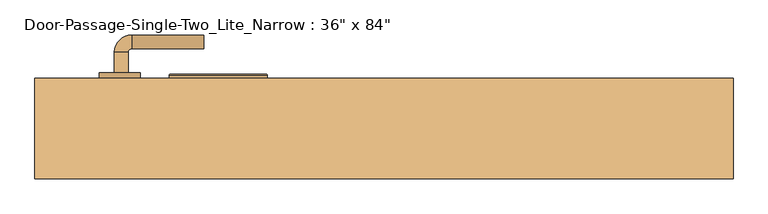
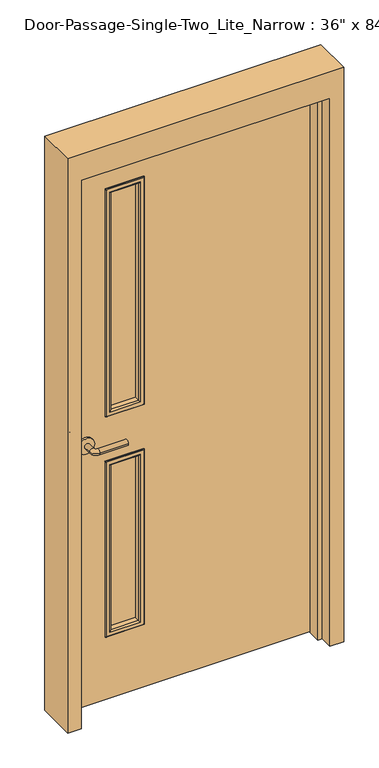
"""IFC4 building model written with IfcOpenShell, lengths in millimetres: door geometry."""

from ifc_helpers import new_model, si_unit, point, frame, frame_2d, origin, place, context, project, spatial, polyline, circle_curve, ellipse_curve, trimmed, segment, composite_curve, outline, extrude, faceted_brep, source, transform, mapped, element, save
from ifc_brep_helpers import plane_surface, cylinder_surface, revolved_surface, advanced_brep


def door_1568ef6f(model_context):
    return source(origin(), model_context, "Body", "SolidModel", [
        advanced_brep(
        [(-392.190625, 4.7, 1016.0), (-372.190625, 4.7, 1016.0), (-372.190625, -25.3, 1016.0), (-392.190625, -25.3, 1016.0), (-367.190625, -30.3, 1016.0), (-367.190625, -50.3, 1016.0), (-262.190625, -50.3, 1016.0), (-262.190625, -30.3, 1016.0)],
        [
            (0, 1, circle_curve(frame((-382.190625, 4.7, 1016.0), z_axis=(0.0, 1.0, 0.0), x_axis=(1.0, 0.0, 0.0)), 10.0)),
            (1, 0, circle_curve(frame((-382.190625, 4.7, 1016.0), z_axis=(0.0, 1.0, 0.0), x_axis=(1.0, 0.0, 0.0)), 10.0)),
            (1, 2),
            (2, 3, circle_curve(frame((-382.190625, -25.3, 1016.0), z_axis=(0.0, 1.0, 0.0), x_axis=(1.0, 0.0, 0.0)), 10.0)),
            (3, 0),
            (3, 2, circle_curve(frame((-382.190625, -25.3, 1016.0), z_axis=(0.0, 1.0, 0.0), x_axis=(1.0, 0.0, 0.0)), 10.0)),
            (4, 5, circle_curve(frame((-367.190625, -40.3, 1016.0), z_axis=(-1.0, 0.0, 0.0), x_axis=(0.0, 1.0, 0.0)), 10.0)),
            (5, 3, circle_curve(frame((-367.190625, -25.3, 1016.0), z_axis=(0.0, 0.0, -1.0), x_axis=(-1.0, 0.0, 0.0)), 25.0)),
            (2, 4, circle_curve(frame((-367.190625, -25.3, 1016.0), z_axis=(0.0, 0.0, 1.0), x_axis=(-1.0, 0.0, 0.0)), 5.0)),
            (5, 4, circle_curve(frame((-367.190625, -40.3, 1016.0), z_axis=(-1.0, 0.0, 0.0), x_axis=(0.0, 1.0, 0.0)), 10.0)),
            (6, 7, circle_curve(frame((-262.190625, -40.3, 1016.0), z_axis=(1.0, 0.0, 0.0), x_axis=(0.0, 1.0, 0.0)), 10.0)),
            (7, 6, circle_curve(frame((-262.190625, -40.3, 1016.0), z_axis=(1.0, 0.0, 0.0), x_axis=(0.0, 1.0, 0.0)), 10.0)),
            (4, 7),
            (6, 5),
        ],
        [
            plane_surface(frame((-382.190625, 4.7, 1016.0), z_axis=(0.0, 1.0, 0.0), x_axis=(0.0, 0.0, 1.0))),
            cylinder_surface(frame((-382.190625, 4.7, 1016.0), z_axis=(0.0, 1.0, 0.0), x_axis=(1.0, 0.0, 0.0)), 10.0),
            revolved_surface(trimmed(ellipse_curve(frame((-382.190625, -25.3, 1016.0), z_axis=(0.0, -1.0, 0.0), x_axis=(1.0, 0.0, 0.0)), 10.0, 10.0), [point((-392.190625, -25.3, 1016.0))], [point((-372.190625, -25.3, 1016.0))], True, "CARTESIAN"), (-367.190625, -25.3, 1016.0), (0.0, 0.0, -1.0)),
            revolved_surface(trimmed(ellipse_curve(frame((-382.190625, -25.3, 1016.0), z_axis=(0.0, -1.0, 0.0), x_axis=(1.0, 0.0, 0.0)), 10.0, 10.0), [point((-372.190625, -25.3, 1016.0))], [point((-392.190625, -25.3, 1016.0))], True, "CARTESIAN"), (-367.190625, -25.3, 1016.0), (0.0, 0.0, -1.0)),
            plane_surface(frame((-262.190625, -40.3, 1016.0), z_axis=(1.0, 0.0, 0.0), x_axis=(0.0, 0.0, 1.0))),
            cylinder_surface(frame((-367.190625, -40.3, 1016.0), z_axis=(-1.0, 0.0, 0.0), x_axis=(0.0, 1.0, 0.0)), 10.0),
        ],
        [
            (0, [[1, 2]]),
            (1, [[3, 4, 5, -2]]),
            (1, [[-5, 6, -3, -1]]),
            (2, [[7, 8, -4, 9]]),
            (3, [[10, -9, -6, -8]]),
            (4, [[11, 12]]),
            (5, [[13, -11, 14, -7]]),
            (5, [[-14, -12, -13, -10]]),
        ],
    ),
        extrude(outline(composite_curve([segment(trimmed(circle_curve(frame_2d((1016.0, -384.690625)), 30.0), [point((1016.0, -414.690625))], [point((1016.0, -354.690625))], False, "CARTESIAN"), True, "CONTINUOUS"), segment(trimmed(circle_curve(frame_2d((1016.0, -384.690625)), 30.0), [point((1016.0, -354.690625))], [point((1016.0, -414.690625))], False, "CARTESIAN"), True, "CONTINUOUS")], self_intersect=False)), frame((0.0, 4.7, 0.0), z_axis=(0.0, 1.0, 0.0), x_axis=(0.0, 0.0, 1.0)), (0.0, 0.0, 1.0), 8.0),
        advanced_brep(
        [(-392.190625, 65.15, 1016.0), (-372.190625, 65.15, 1016.0), (-392.190625, 95.15, 1016.0), (-372.190625, 95.15, 1016.0), (-367.190625, 100.15, 1016.0), (-367.190625, 120.15, 1016.0), (-262.190625, 120.15, 1016.0), (-262.190625, 100.15, 1016.0)],
        [
            (0, 1, circle_curve(frame((-382.190625, 65.15, 1016.0), z_axis=(0.0, -1.0, 0.0), x_axis=(1.0, 0.0, 0.0)), 10.0)),
            (1, 0, circle_curve(frame((-382.190625, 65.15, 1016.0), z_axis=(0.0, -1.0, 0.0), x_axis=(1.0, 0.0, 0.0)), 10.0)),
            (0, 2),
            (2, 3, circle_curve(frame((-382.190625, 95.15, 1016.0), z_axis=(0.0, -1.0, 0.0), x_axis=(1.0, 0.0, 0.0)), 10.0)),
            (3, 1),
            (3, 2, circle_curve(frame((-382.190625, 95.15, 1016.0), z_axis=(0.0, -1.0, 0.0), x_axis=(1.0, 0.0, 0.0)), 10.0)),
            (4, 3, circle_curve(frame((-367.190625, 95.15, 1016.0), z_axis=(0.0, 0.0, 1.0), x_axis=(-1.0, 0.0, 0.0)), 5.0)),
            (2, 5, circle_curve(frame((-367.190625, 95.15, 1016.0), z_axis=(0.0, 0.0, -1.0), x_axis=(-1.0, 0.0, 0.0)), 25.0)),
            (5, 4, circle_curve(frame((-367.190625, 110.15, 1016.0), z_axis=(-1.0, 0.0, 0.0), x_axis=(0.0, -1.0, 0.0)), 10.0)),
            (4, 5, circle_curve(frame((-367.190625, 110.15, 1016.0), z_axis=(-1.0, 0.0, 0.0), x_axis=(0.0, -1.0, 0.0)), 10.0)),
            (6, 7, circle_curve(frame((-262.190625, 110.15, 1016.0), z_axis=(1.0, 0.0, 0.0), x_axis=(0.0, -1.0, 0.0)), 10.0)),
            (7, 6, circle_curve(frame((-262.190625, 110.15, 1016.0), z_axis=(1.0, 0.0, 0.0), x_axis=(0.0, -1.0, 0.0)), 10.0)),
            (5, 6),
            (7, 4),
        ],
        [
            plane_surface(frame((-382.190625, 65.15, 1016.0), z_axis=(0.0, -1.0, 0.0), x_axis=(0.0, 0.0, 1.0))),
            cylinder_surface(frame((-382.190625, 65.15, 1016.0), z_axis=(0.0, -1.0, 0.0), x_axis=(1.0, 0.0, 0.0)), 10.0),
            revolved_surface(trimmed(ellipse_curve(frame((-382.190625, 95.15, 1016.0), z_axis=(0.0, -1.0, 0.0), x_axis=(1.0, 0.0, 0.0)), 10.0, 10.0), [point((-392.190625, 95.15, 1016.0))], [point((-372.190625, 95.15, 1016.0))], True, "CARTESIAN"), (-367.190625, 95.15, 1016.0), (0.0, 0.0, -1.0)),
            revolved_surface(trimmed(ellipse_curve(frame((-382.190625, 95.15, 1016.0), z_axis=(0.0, -1.0, 0.0), x_axis=(1.0, 0.0, 0.0)), 10.0, 10.0), [point((-372.190625, 95.15, 1016.0))], [point((-392.190625, 95.15, 1016.0))], True, "CARTESIAN"), (-367.190625, 95.15, 1016.0), (0.0, 0.0, -1.0)),
            plane_surface(frame((-262.190625, 110.15, 1016.0), z_axis=(1.0, 0.0, 0.0), x_axis=(0.0, 0.0, 1.0))),
            cylinder_surface(frame((-367.190625, 110.15, 1016.0), z_axis=(-1.0, 0.0, 0.0), x_axis=(0.0, -1.0, 0.0)), 10.0),
        ],
        [
            (0, [[1, 2]]),
            (1, [[-1, 3, 4, 5]]),
            (1, [[-2, -5, 6, -3]]),
            (2, [[7, -4, 8, 9]]),
            (3, [[-8, -6, -7, 10]]),
            (4, [[11, 12]]),
            (5, [[-9, 13, -12, 14]]),
            (5, [[-10, -14, -11, -13]]),
        ],
    ),
        extrude(outline(composite_curve([segment(trimmed(circle_curve(frame_2d((1016.0, -384.690625)), 30.0), [point((1016.0, -414.690625))], [point((1016.0, -354.690625))], False, "CARTESIAN"), True, "CONTINUOUS"), segment(trimmed(circle_curve(frame_2d((1016.0, -384.690625)), 30.0), [point((1016.0, -354.690625))], [point((1016.0, -414.690625))], False, "CARTESIAN"), True, "CONTINUOUS")], self_intersect=False)), frame((0.0, 57.15, 0.0), z_axis=(0.0, 1.0, 0.0), x_axis=(0.0, 0.0, 1.0)), (0.0, 0.0, 1.0), 8.0),
        faceted_brep([(457.2, 7.9375, 0.0), (457.2, 57.15, 0.0), (508.0, 57.15, 0.0), (508.0, -88.9, 0.0), (457.2, -88.9, 0.0), (457.2, -39.6875, 0.0), (441.325, -39.6875, 0.0), (441.325, 7.9375, 0.0), (457.2, 7.9375, 2133.6), (457.2, 57.15, 2133.6), (-457.2, 57.15, 2133.6), (-457.2, 57.15, 0.0), (-508.0, 57.15, 0.0), (-508.0, 57.15, 2235.2), (508.0, 57.15, 2235.2), (508.0, -88.9, 2235.2), (-508.0, -88.9, 2235.2), (-508.0, -88.9, 0.0), (-457.2, -88.9, 0.0), (-457.2, -88.9, 2133.6), (457.2, -88.9, 2133.6), (457.2, -39.6875, 2133.6), (-457.2, -39.6875, 2133.6), (-457.2, -39.6875, 0.0), (-441.325, -39.6875, 0.0), (-441.325, -39.6875, 2117.725), (441.325, -39.6875, 2117.725), (441.325, 7.9375, 2117.725), (-441.325, 7.9375, 2117.725), (-441.325, 7.9375, 0.0), (-457.2, 7.9375, 0.0), (-457.2, 7.9375, 2133.6)], [[[0, 1, 2, 3, 4, 5, 6, 7]], [[1, 0, 8, 9]], [[2, 1, 9, 10, 11, 12, 13, 14]], [[3, 2, 14, 15]], [[4, 3, 15, 16, 17, 18, 19, 20]], [[5, 4, 20, 21]], [[6, 5, 21, 22, 23, 24, 25, 26]], [[7, 6, 26, 27]], [[0, 7, 27, 28, 29, 30, 31, 8]], [[9, 8, 31, 10]], [[20, 19, 22, 21]], [[26, 25, 28, 27]], [[12, 11, 30, 29, 24, 23, 18, 17]], [[11, 10, 31, 30]], [[13, 12, 17, 16]], [[19, 18, 23, 22]], [[25, 24, 29, 28]], [[15, 14, 13, 16]]]),
        extrude(outline(polyline([(2133.6, -457.2), (0.0, -457.2), (0.0, 457.2), (2133.6, 457.2), (2133.6, -457.2)]), holes=[polyline([(1981.2, -304.8), (1981.2, -177.8), (1111.25, -177.8), (1111.25, -304.8), (1981.2, -304.8)]), polyline([(920.75, -304.8), (920.75, -177.8), (254.0, -177.8), (254.0, -304.8), (920.75, -304.8)])]), frame((0.0, 12.7, 0.0), z_axis=(0.0, 1.0, 0.0), x_axis=(0.0, 0.0, 1.0)), (0.0, 0.0, 1.0), 44.45),
        extrude(outline(polyline([(-177.8, 31.75), (-304.8, 31.75), (-304.8, 38.1), (-177.8, 38.1), (-177.8, 31.75)])), frame((0.0, 0.0, 1111.25), z_axis=(0.0, 0.0, 1.0), x_axis=(1.0, 0.0, 0.0)), (0.0, 0.0, 1.0), 869.95),
        extrude(outline(polyline([(-177.8, 31.75), (-304.8, 31.75), (-304.8, 38.1), (-177.8, 38.1), (-177.8, 31.75)])), frame((0.0, 0.0, 254.0), z_axis=(0.0, 0.0, 1.0), x_axis=(1.0, 0.0, 0.0)), (0.0, 0.0, 1.0), 666.75),
        advanced_brep(
        [(-177.8, 31.75, 920.75), (-177.8, 12.7, 920.75), (-177.8, 12.7, 254.0), (-177.8, 31.75, 254.0), (-189.8, 11.7, 908.75), (-189.8, 31.75, 908.75), (-189.8, 31.75, 266.0), (-189.8, 11.7, 266.0), (-184.8, 6.7, 913.75), (-184.8, 6.7, 261.0), (-169.8, 8.7, 928.75), (-171.8, 6.7, 926.75), (-171.8, 6.7, 248.0), (-169.8, 8.7, 246.0), (-169.8, 12.7, 928.75), (-169.8, 12.7, 246.0), (-304.8, 12.7, 254.0), (-304.8, 31.75, 254.0), (-292.8, 31.75, 266.0), (-292.8, 11.7, 266.0), (-297.8, 6.7, 261.0), (-310.8, 6.7, 248.0), (-312.8, 8.7, 246.0), (-312.8, 12.7, 246.0), (-304.8, 12.7, 920.75), (-304.8, 31.75, 920.75), (-292.8, 31.75, 908.75), (-292.8, 11.7, 908.75), (-297.8, 6.7, 913.75), (-310.8, 6.7, 926.75), (-312.8, 8.7, 928.75), (-312.8, 12.7, 928.75)],
        [
            (0, 1),
            (1, 2),
            (2, 3),
            (3, 0),
            (4, 5),
            (5, 6),
            (6, 7),
            (7, 4),
            (8, 4, ellipse_curve(frame((-184.8, 11.7, 913.75), z_axis=(0.7071067811865475, 0.0, -0.7071067811865475), x_axis=(0.7071067811865474, 0.0, 0.7071067811865476)), 7.0710678, 5.0)),
            (7, 9, ellipse_curve(frame((-184.8, 11.7, 261.0), z_axis=(0.7071067811865475, 0.0, 0.7071067811865475), x_axis=(-0.7071067811865474, 0.0, 0.7071067811865476)), 7.0710678, 5.0)),
            (9, 8),
            (10, 11, ellipse_curve(frame((-171.8, 8.7, 926.75), z_axis=(0.7071067811865475, 0.0, -0.7071067811865475), x_axis=(0.7071067811865474, 0.0, 0.7071067811865476)), 2.8284271, 2.0)),
            (11, 12),
            (12, 13, ellipse_curve(frame((-171.8, 8.7, 248.0), z_axis=(0.7071067811865475, 0.0, 0.7071067811865475), x_axis=(-0.7071067811865474, 0.0, 0.7071067811865476)), 2.8284271, 2.0)),
            (13, 10),
            (14, 10),
            (13, 15),
            (15, 14),
            (2, 16),
            (16, 17),
            (17, 3),
            (6, 18),
            (18, 19),
            (19, 7),
            (19, 20, ellipse_curve(frame((-297.8, 11.7, 261.0), z_axis=(0.7071067811865475, 0.0, -0.7071067811865475), x_axis=(0.7071067811865476, 0.0, 0.7071067811865474)), 7.0710678, 5.0)),
            (20, 9),
            (12, 21),
            (21, 22, ellipse_curve(frame((-310.8, 8.7, 248.0), z_axis=(0.7071067811865475, 0.0, -0.7071067811865475), x_axis=(0.7071067811865476, 0.0, 0.7071067811865474)), 2.8284271, 2.0)),
            (22, 13),
            (22, 23),
            (23, 15),
            (16, 24),
            (24, 25),
            (25, 17),
            (18, 26),
            (26, 27),
            (27, 19),
            (27, 28, ellipse_curve(frame((-297.8, 11.7, 913.75), z_axis=(-0.7071067811865475, 0.0, -0.7071067811865475), x_axis=(0.7071067811865474, 0.0, -0.7071067811865476)), 7.0710678, 5.0)),
            (28, 20),
            (21, 29),
            (29, 30, ellipse_curve(frame((-310.8, 8.7, 926.75), z_axis=(-0.7071067811865475, 0.0, -0.7071067811865475), x_axis=(0.7071067811865474, 0.0, -0.7071067811865476)), 2.8284271, 2.0)),
            (30, 22),
            (30, 31),
            (31, 23),
            (31, 14),
            (1, 24),
            (0, 25),
            (5, 26),
            (4, 27),
            (8, 28),
            (11, 29),
            (10, 30),
        ],
        [
            plane_surface(frame((-177.8, 12.7, 920.75), z_axis=(1.0, 0.0, 0.0), x_axis=(0.0, 0.0, -1.0))),
            plane_surface(frame((-189.8, 31.75, 908.75), z_axis=(-1.0, 0.0, 0.0), x_axis=(0.0, 0.0, -1.0))),
            cylinder_surface(frame((-184.8, 11.7, 920.75), z_axis=(0.0, 0.0, 1.0), x_axis=(1.0, 0.0, 0.0)), 5.0),
            cylinder_surface(frame((-171.8, 8.7, 920.75), z_axis=(0.0, 0.0, 1.0), x_axis=(1.0, 0.0, 0.0)), 2.0),
            plane_surface(frame((-169.8, 8.7, 928.75), z_axis=(1.0, 0.0, 0.0), x_axis=(0.0, 0.0, -1.0))),
            plane_surface(frame((-177.8, 12.7, 254.0), z_axis=(0.0, 0.0, -1.0), x_axis=(-1.0, 0.0, 0.0))),
            plane_surface(frame((-189.8, 31.75, 266.0), z_axis=(0.0, 0.0, 1.0), x_axis=(-1.0, 0.0, 0.0))),
            cylinder_surface(frame((-177.8, 11.7, 261.0), z_axis=(1.0, 0.0, 0.0), x_axis=(0.0, 0.0, -1.0)), 5.0),
            cylinder_surface(frame((-177.8, 8.7, 248.0), z_axis=(1.0, 0.0, 0.0), x_axis=(0.0, 0.0, -1.0)), 2.0),
            plane_surface(frame((-169.8, 8.7, 246.0), z_axis=(0.0, 0.0, -1.0), x_axis=(-1.0, 0.0, 0.0))),
            plane_surface(frame((-304.8, 12.7, 254.0), z_axis=(-1.0, 0.0, 0.0), x_axis=(0.0, 0.0, 1.0))),
            plane_surface(frame((-292.8, 31.75, 266.0), z_axis=(1.0, 0.0, 0.0), x_axis=(0.0, 0.0, 1.0))),
            cylinder_surface(frame((-297.8, 11.7, 254.0), z_axis=(0.0, 0.0, -1.0), x_axis=(-1.0, 0.0, 0.0)), 5.0),
            cylinder_surface(frame((-310.8, 8.7, 254.0), z_axis=(0.0, 0.0, -1.0), x_axis=(-1.0, 0.0, 0.0)), 2.0),
            plane_surface(frame((-312.8, 8.7, 246.0), z_axis=(-1.0, 0.0, 0.0), x_axis=(0.0, 0.0, 1.0))),
            plane_surface(frame((-312.8, 12.7, 928.75), z_axis=(0.0, 1.0, 0.0), x_axis=(1.0, 0.0, 0.0))),
            plane_surface(frame((-304.8, 12.7, 920.75), z_axis=(0.0, 0.0, 1.0), x_axis=(1.0, 0.0, 0.0))),
            plane_surface(frame((-304.8, 31.75, 920.75), z_axis=(0.0, 1.0, 0.0), x_axis=(1.0, 0.0, 0.0))),
            plane_surface(frame((-292.8, 31.75, 908.75), z_axis=(0.0, 0.0, -1.0), x_axis=(1.0, 0.0, 0.0))),
            cylinder_surface(frame((-304.8, 11.7, 913.75), z_axis=(-1.0, 0.0, 0.0), x_axis=(0.0, 0.0, 1.0)), 5.0),
            plane_surface(frame((-297.8, 6.7, 913.75), z_axis=(0.0, -1.0, 0.0), x_axis=(1.0, 0.0, 0.0))),
            cylinder_surface(frame((-304.8, 8.7, 926.75), z_axis=(-1.0, 0.0, 0.0), x_axis=(0.0, 0.0, 1.0)), 2.0),
            plane_surface(frame((-312.8, 8.7, 928.75), z_axis=(0.0, 0.0, 1.0), x_axis=(1.0, 0.0, 0.0))),
        ],
        [
            (0, [[1, 2, 3, 4]]),
            (1, [[5, 6, 7, 8]]),
            (2, [[9, -8, 10, 11]]),
            (3, [[12, 13, 14, 15]]),
            (4, [[16, -15, 17, 18]]),
            (5, [[-3, 19, 20, 21]]),
            (6, [[-7, 22, 23, 24]]),
            (7, [[-10, -24, 25, 26]]),
            (8, [[-14, 27, 28, 29]]),
            (9, [[-17, -29, 30, 31]]),
            (10, [[-20, 32, 33, 34]]),
            (11, [[-23, 35, 36, 37]]),
            (12, [[-25, -37, 38, 39]]),
            (13, [[-28, 40, 41, 42]]),
            (14, [[-30, -42, 43, 44]]),
            (15, [[-31, -44, 45, -18], [46, -32, -19, -2]]),
            (16, [[-33, -46, -1, 47]]),
            (17, [[-21, -34, -47, -4], [48, -35, -22, -6]]),
            (18, [[-36, -48, -5, 49]]),
            (19, [[-38, -49, -9, 50]]),
            (20, [[51, -40, -27, -13], [-26, -39, -50, -11]]),
            (21, [[-41, -51, -12, 52]]),
            (22, [[-43, -52, -16, -45]]),
        ],
    ),
        advanced_brep(
        [(-304.8, 38.1, 920.75), (-304.8, 57.15, 920.75), (-304.8, 57.15, 254.0), (-304.8, 38.1, 254.0), (-292.8, 58.15, 908.75), (-292.8, 38.1, 908.75), (-292.8, 38.1, 266.0), (-292.8, 58.15, 266.0), (-297.8, 63.15, 913.75), (-297.8, 63.15, 261.0), (-312.8, 61.15, 928.75), (-310.8, 63.15, 926.75), (-310.8, 63.15, 248.0), (-312.8, 61.15, 246.0), (-312.8, 57.15, 928.75), (-312.8, 57.15, 246.0), (-177.8, 57.15, 254.0), (-177.8, 38.1, 254.0), (-189.8, 38.1, 266.0), (-189.8, 58.15, 266.0), (-184.8, 63.15, 261.0), (-171.8, 63.15, 248.0), (-169.8, 61.15, 246.0), (-169.8, 57.15, 246.0), (-177.8, 57.15, 920.75), (-177.8, 38.1, 920.75), (-189.8, 38.1, 908.75), (-189.8, 58.15, 908.75), (-184.8, 63.15, 913.75), (-171.8, 63.15, 926.75), (-169.8, 61.15, 928.75), (-169.8, 57.15, 928.75)],
        [
            (0, 1),
            (1, 2),
            (2, 3),
            (3, 0),
            (4, 5),
            (5, 6),
            (6, 7),
            (7, 4),
            (8, 4, ellipse_curve(frame((-297.8, 58.15, 913.75), z_axis=(-0.7071067811865475, 0.0, -0.7071067811865475), x_axis=(-0.7071067811865474, 0.0, 0.7071067811865476)), 7.0710678, 5.0)),
            (7, 9, ellipse_curve(frame((-297.8, 58.15, 261.0), z_axis=(-0.7071067811865475, 0.0, 0.7071067811865475), x_axis=(0.7071067811865474, 0.0, 0.7071067811865476)), 7.0710678, 5.0)),
            (9, 8),
            (10, 11, ellipse_curve(frame((-310.8, 61.15, 926.75), z_axis=(-0.7071067811865475, 0.0, -0.7071067811865475), x_axis=(-0.7071067811865474, 0.0, 0.7071067811865476)), 2.8284271, 2.0)),
            (11, 12),
            (12, 13, ellipse_curve(frame((-310.8, 61.15, 248.0), z_axis=(-0.7071067811865475, 0.0, 0.7071067811865475), x_axis=(0.7071067811865474, 0.0, 0.7071067811865476)), 2.8284271, 2.0)),
            (13, 10),
            (14, 10),
            (13, 15),
            (15, 14),
            (2, 16),
            (16, 17),
            (17, 3),
            (6, 18),
            (18, 19),
            (19, 7),
            (19, 20, ellipse_curve(frame((-184.8, 58.15, 261.0), z_axis=(-0.7071067811865475, 0.0, -0.7071067811865475), x_axis=(-0.7071067811865476, 0.0, 0.7071067811865474)), 7.0710678, 5.0)),
            (20, 9),
            (12, 21),
            (21, 22, ellipse_curve(frame((-171.8, 61.15, 248.0), z_axis=(-0.7071067811865475, 0.0, -0.7071067811865475), x_axis=(-0.7071067811865476, 0.0, 0.7071067811865474)), 2.8284271, 2.0)),
            (22, 13),
            (22, 23),
            (23, 15),
            (16, 24),
            (24, 25),
            (25, 17),
            (18, 26),
            (26, 27),
            (27, 19),
            (27, 28, ellipse_curve(frame((-184.8, 58.15, 913.75), z_axis=(0.7071067811865475, 0.0, -0.7071067811865475), x_axis=(-0.7071067811865474, 0.0, -0.7071067811865476)), 7.0710678, 5.0)),
            (28, 20),
            (21, 29),
            (29, 30, ellipse_curve(frame((-171.8, 61.15, 926.75), z_axis=(0.7071067811865475, 0.0, -0.7071067811865475), x_axis=(-0.7071067811865474, 0.0, -0.7071067811865476)), 2.8284271, 2.0)),
            (30, 22),
            (30, 31),
            (31, 23),
            (31, 14),
            (1, 24),
            (0, 25),
            (5, 26),
            (4, 27),
            (8, 28),
            (11, 29),
            (10, 30),
        ],
        [
            plane_surface(frame((-304.8, 57.15, 920.75), z_axis=(-1.0, 0.0, 0.0), x_axis=(0.0, 0.0, -1.0))),
            plane_surface(frame((-292.8, 38.1, 908.75), z_axis=(1.0, 0.0, 0.0), x_axis=(0.0, 0.0, -1.0))),
            cylinder_surface(frame((-297.8, 58.15, 920.75), z_axis=(0.0, 0.0, 1.0), x_axis=(-1.0, 0.0, 0.0)), 5.0),
            cylinder_surface(frame((-310.8, 61.15, 920.75), z_axis=(0.0, 0.0, 1.0), x_axis=(-1.0, 0.0, 0.0)), 2.0),
            plane_surface(frame((-312.8, 61.15, 928.75), z_axis=(-1.0, 0.0, 0.0), x_axis=(0.0, 0.0, -1.0))),
            plane_surface(frame((-304.8, 57.15, 254.0), z_axis=(0.0, 0.0, -1.0), x_axis=(1.0, 0.0, 0.0))),
            plane_surface(frame((-292.8, 38.1, 266.0), z_axis=(0.0, 0.0, 1.0), x_axis=(1.0, 0.0, 0.0))),
            cylinder_surface(frame((-304.8, 58.15, 261.0), z_axis=(-1.0, 0.0, 0.0), x_axis=(0.0, 0.0, -1.0)), 5.0),
            cylinder_surface(frame((-304.8, 61.15, 248.0), z_axis=(-1.0, 0.0, 0.0), x_axis=(0.0, 0.0, -1.0)), 2.0),
            plane_surface(frame((-312.8, 61.15, 246.0), z_axis=(0.0, 0.0, -1.0), x_axis=(1.0, 0.0, 0.0))),
            plane_surface(frame((-177.8, 57.15, 254.0), z_axis=(1.0, 0.0, 0.0), x_axis=(0.0, 0.0, 1.0))),
            plane_surface(frame((-189.8, 38.1, 266.0), z_axis=(-1.0, 0.0, 0.0), x_axis=(0.0, 0.0, 1.0))),
            cylinder_surface(frame((-184.8, 58.15, 254.0), z_axis=(0.0, 0.0, -1.0), x_axis=(1.0, 0.0, 0.0)), 5.0),
            cylinder_surface(frame((-171.8, 61.15, 254.0), z_axis=(0.0, 0.0, -1.0), x_axis=(1.0, 0.0, 0.0)), 2.0),
            plane_surface(frame((-169.8, 61.15, 246.0), z_axis=(1.0, 0.0, 0.0), x_axis=(0.0, 0.0, 1.0))),
            plane_surface(frame((-169.8, 57.15, 928.75), z_axis=(0.0, -1.0, 0.0), x_axis=(-1.0, 0.0, 0.0))),
            plane_surface(frame((-177.8, 57.15, 920.75), z_axis=(0.0, 0.0, 1.0), x_axis=(-1.0, 0.0, 0.0))),
            plane_surface(frame((-177.8, 38.1, 920.75), z_axis=(0.0, -1.0, 0.0), x_axis=(-1.0, 0.0, 0.0))),
            plane_surface(frame((-189.8, 38.1, 908.75), z_axis=(0.0, 0.0, -1.0), x_axis=(-1.0, 0.0, 0.0))),
            cylinder_surface(frame((-177.8, 58.15, 913.75), z_axis=(1.0, 0.0, 0.0), x_axis=(0.0, 0.0, 1.0)), 5.0),
            plane_surface(frame((-184.8, 63.15, 913.75), z_axis=(0.0, 1.0, 0.0), x_axis=(-1.0, 0.0, 0.0))),
            cylinder_surface(frame((-177.8, 61.15, 926.75), z_axis=(1.0, 0.0, 0.0), x_axis=(0.0, 0.0, 1.0)), 2.0),
            plane_surface(frame((-169.8, 61.15, 928.75), z_axis=(0.0, 0.0, 1.0), x_axis=(-1.0, 0.0, 0.0))),
        ],
        [
            (0, [[1, 2, 3, 4]]),
            (1, [[5, 6, 7, 8]]),
            (2, [[9, -8, 10, 11]]),
            (3, [[12, 13, 14, 15]]),
            (4, [[16, -15, 17, 18]]),
            (5, [[-3, 19, 20, 21]]),
            (6, [[-7, 22, 23, 24]]),
            (7, [[-10, -24, 25, 26]]),
            (8, [[-14, 27, 28, 29]]),
            (9, [[-17, -29, 30, 31]]),
            (10, [[-20, 32, 33, 34]]),
            (11, [[-23, 35, 36, 37]]),
            (12, [[-25, -37, 38, 39]]),
            (13, [[-28, 40, 41, 42]]),
            (14, [[-30, -42, 43, 44]]),
            (15, [[-31, -44, 45, -18], [46, -32, -19, -2]]),
            (16, [[-33, -46, -1, 47]]),
            (17, [[-21, -34, -47, -4], [48, -35, -22, -6]]),
            (18, [[-36, -48, -5, 49]]),
            (19, [[-38, -49, -9, 50]]),
            (20, [[51, -40, -27, -13], [-26, -39, -50, -11]]),
            (21, [[-41, -51, -12, 52]]),
            (22, [[-43, -52, -16, -45]]),
        ],
    ),
        advanced_brep(
        [(-304.8, 31.75, 1111.25), (-304.8, 12.7, 1111.25), (-304.8, 12.7, 1981.2), (-304.8, 31.75, 1981.2), (-292.8, 11.7, 1123.25), (-292.8, 31.75, 1123.25), (-292.8, 31.75, 1969.2), (-292.8, 11.7, 1969.2), (-297.8, 6.7, 1118.25), (-297.8, 6.7, 1974.2), (-312.8, 8.7, 1103.25), (-310.8, 6.7, 1105.25), (-310.8, 6.7, 1987.2), (-312.8, 8.7, 1989.2), (-312.8, 12.7, 1103.25), (-312.8, 12.7, 1989.2), (-177.8, 12.7, 1981.2), (-177.8, 31.75, 1981.2), (-189.8, 31.75, 1969.2), (-189.8, 11.7, 1969.2), (-184.8, 6.7, 1974.2), (-171.8, 6.7, 1987.2), (-169.8, 8.7, 1989.2), (-169.8, 12.7, 1989.2), (-177.8, 12.7, 1111.25), (-177.8, 31.75, 1111.25), (-189.8, 31.75, 1123.25), (-189.8, 11.7, 1123.25), (-184.8, 6.7, 1118.25), (-171.8, 6.7, 1105.25), (-169.8, 8.7, 1103.25), (-169.8, 12.7, 1103.25)],
        [
            (0, 1),
            (1, 2),
            (2, 3),
            (3, 0),
            (4, 5),
            (5, 6),
            (6, 7),
            (7, 4),
            (8, 4, ellipse_curve(frame((-297.8, 11.7, 1118.25), z_axis=(-0.7071067811865475, 0.0, 0.7071067811865475), x_axis=(-0.7071067811865474, 0.0, -0.7071067811865476)), 7.0710678, 5.0)),
            (7, 9, ellipse_curve(frame((-297.8, 11.7, 1974.2), z_axis=(-0.7071067811865475, 0.0, -0.7071067811865475), x_axis=(0.7071067811865474, 0.0, -0.7071067811865476)), 7.0710678, 5.0)),
            (9, 8),
            (10, 11, ellipse_curve(frame((-310.8, 8.7, 1105.25), z_axis=(-0.7071067811865475, 0.0, 0.7071067811865475), x_axis=(-0.7071067811865474, 0.0, -0.7071067811865476)), 2.8284271, 2.0)),
            (11, 12),
            (12, 13, ellipse_curve(frame((-310.8, 8.7, 1987.2), z_axis=(-0.7071067811865475, 0.0, -0.7071067811865475), x_axis=(0.7071067811865474, 0.0, -0.7071067811865476)), 2.8284271, 2.0)),
            (13, 10),
            (14, 10),
            (13, 15),
            (15, 14),
            (2, 16),
            (16, 17),
            (17, 3),
            (6, 18),
            (18, 19),
            (19, 7),
            (19, 20, ellipse_curve(frame((-184.8, 11.7, 1974.2), z_axis=(-0.7071067811865475, 0.0, 0.7071067811865475), x_axis=(-0.7071067811865476, 0.0, -0.7071067811865474)), 7.0710678, 5.0)),
            (20, 9),
            (12, 21),
            (21, 22, ellipse_curve(frame((-171.8, 8.7, 1987.2), z_axis=(-0.7071067811865475, 0.0, 0.7071067811865475), x_axis=(-0.7071067811865476, 0.0, -0.7071067811865474)), 2.8284271, 2.0)),
            (22, 13),
            (22, 23),
            (23, 15),
            (16, 24),
            (24, 25),
            (25, 17),
            (18, 26),
            (26, 27),
            (27, 19),
            (27, 28, ellipse_curve(frame((-184.8, 11.7, 1118.25), z_axis=(0.7071067811865475, 0.0, 0.7071067811865475), x_axis=(-0.7071067811865474, 0.0, 0.7071067811865476)), 7.0710678, 5.0)),
            (28, 20),
            (21, 29),
            (29, 30, ellipse_curve(frame((-171.8, 8.7, 1105.25), z_axis=(0.7071067811865475, 0.0, 0.7071067811865475), x_axis=(-0.7071067811865474, 0.0, 0.7071067811865476)), 2.8284271, 2.0)),
            (30, 22),
            (30, 31),
            (31, 23),
            (31, 14),
            (1, 24),
            (0, 25),
            (5, 26),
            (4, 27),
            (8, 28),
            (11, 29),
            (10, 30),
        ],
        [
            plane_surface(frame((-304.8, 12.7, 1111.25), z_axis=(-1.0, 0.0, 0.0), x_axis=(0.0, 0.0, 1.0))),
            plane_surface(frame((-292.8, 31.75, 1123.25), z_axis=(1.0, 0.0, 0.0), x_axis=(0.0, 0.0, 1.0))),
            cylinder_surface(frame((-297.8, 11.7, 1111.25), z_axis=(0.0, 0.0, -1.0), x_axis=(-1.0, 0.0, 0.0)), 5.0),
            cylinder_surface(frame((-310.8, 8.7, 1111.25), z_axis=(0.0, 0.0, -1.0), x_axis=(-1.0, 0.0, 0.0)), 2.0),
            plane_surface(frame((-312.8, 8.7, 1103.25), z_axis=(-1.0, 0.0, 0.0), x_axis=(0.0, 0.0, 1.0))),
            plane_surface(frame((-304.8, 12.7, 1981.2), z_axis=(0.0, 0.0, 1.0), x_axis=(1.0, 0.0, 0.0))),
            plane_surface(frame((-292.8, 31.75, 1969.2), z_axis=(0.0, 0.0, -1.0), x_axis=(1.0, 0.0, 0.0))),
            cylinder_surface(frame((-304.8, 11.7, 1974.2), z_axis=(-1.0, 0.0, 0.0), x_axis=(0.0, 0.0, 1.0)), 5.0),
            cylinder_surface(frame((-304.8, 8.7, 1987.2), z_axis=(-1.0, 0.0, 0.0), x_axis=(0.0, 0.0, 1.0)), 2.0),
            plane_surface(frame((-312.8, 8.7, 1989.2), z_axis=(0.0, 0.0, 1.0), x_axis=(1.0, 0.0, 0.0))),
            plane_surface(frame((-177.8, 12.7, 1981.2), z_axis=(1.0, 0.0, 0.0), x_axis=(0.0, 0.0, -1.0))),
            plane_surface(frame((-189.8, 31.75, 1969.2), z_axis=(-1.0, 0.0, 0.0), x_axis=(0.0, 0.0, -1.0))),
            cylinder_surface(frame((-184.8, 11.7, 1981.2), z_axis=(0.0, 0.0, 1.0), x_axis=(1.0, 0.0, 0.0)), 5.0),
            cylinder_surface(frame((-171.8, 8.7, 1981.2), z_axis=(0.0, 0.0, 1.0), x_axis=(1.0, 0.0, 0.0)), 2.0),
            plane_surface(frame((-169.8, 8.7, 1989.2), z_axis=(1.0, 0.0, 0.0), x_axis=(0.0, 0.0, -1.0))),
            plane_surface(frame((-169.8, 12.7, 1103.25), z_axis=(0.0, 1.0, 0.0), x_axis=(-1.0, 0.0, 0.0))),
            plane_surface(frame((-177.8, 12.7, 1111.25), z_axis=(0.0, 0.0, -1.0), x_axis=(-1.0, 0.0, 0.0))),
            plane_surface(frame((-177.8, 31.75, 1111.25), z_axis=(0.0, 1.0, 0.0), x_axis=(-1.0, 0.0, 0.0))),
            plane_surface(frame((-189.8, 31.75, 1123.25), z_axis=(0.0, 0.0, 1.0), x_axis=(-1.0, 0.0, 0.0))),
            cylinder_surface(frame((-177.8, 11.7, 1118.25), z_axis=(1.0, 0.0, 0.0), x_axis=(0.0, 0.0, -1.0)), 5.0),
            plane_surface(frame((-184.8, 6.7, 1118.25), z_axis=(0.0, -1.0, 0.0), x_axis=(-1.0, 0.0, 0.0))),
            cylinder_surface(frame((-177.8, 8.7, 1105.25), z_axis=(1.0, 0.0, 0.0), x_axis=(0.0, 0.0, -1.0)), 2.0),
            plane_surface(frame((-169.8, 8.7, 1103.25), z_axis=(0.0, 0.0, -1.0), x_axis=(-1.0, 0.0, 0.0))),
        ],
        [
            (0, [[1, 2, 3, 4]]),
            (1, [[5, 6, 7, 8]]),
            (2, [[9, -8, 10, 11]]),
            (3, [[12, 13, 14, 15]]),
            (4, [[16, -15, 17, 18]]),
            (5, [[-3, 19, 20, 21]]),
            (6, [[-7, 22, 23, 24]]),
            (7, [[-10, -24, 25, 26]]),
            (8, [[-14, 27, 28, 29]]),
            (9, [[-17, -29, 30, 31]]),
            (10, [[-20, 32, 33, 34]]),
            (11, [[-23, 35, 36, 37]]),
            (12, [[-25, -37, 38, 39]]),
            (13, [[-28, 40, 41, 42]]),
            (14, [[-30, -42, 43, 44]]),
            (15, [[-31, -44, 45, -18], [46, -32, -19, -2]]),
            (16, [[-33, -46, -1, 47]]),
            (17, [[-21, -34, -47, -4], [48, -35, -22, -6]]),
            (18, [[-36, -48, -5, 49]]),
            (19, [[-38, -49, -9, 50]]),
            (20, [[51, -40, -27, -13], [-26, -39, -50, -11]]),
            (21, [[-41, -51, -12, 52]]),
            (22, [[-43, -52, -16, -45]]),
        ],
    ),
        advanced_brep(
        [(-304.8, 38.1, 1981.2), (-304.8, 57.15, 1981.2), (-304.8, 57.15, 1111.25), (-304.8, 38.1, 1111.25), (-292.8, 58.15, 1969.2), (-292.8, 38.1, 1969.2), (-292.8, 38.1, 1123.25), (-292.8, 58.15, 1123.25), (-297.8, 63.15, 1974.2), (-297.8, 63.15, 1118.25), (-312.8, 61.15, 1989.2), (-310.8, 63.15, 1987.2), (-310.8, 63.15, 1105.25), (-312.8, 61.15, 1103.25), (-312.8, 57.15, 1989.2), (-312.8, 57.15, 1103.25), (-177.8, 57.15, 1111.25), (-177.8, 38.1, 1111.25), (-189.8, 38.1, 1123.25), (-189.8, 58.15, 1123.25), (-184.8, 63.15, 1118.25), (-171.8, 63.15, 1105.25), (-169.8, 61.15, 1103.25), (-169.8, 57.15, 1103.25), (-177.8, 57.15, 1981.2), (-177.8, 38.1, 1981.2), (-189.8, 38.1, 1969.2), (-189.8, 58.15, 1969.2), (-184.8, 63.15, 1974.2), (-171.8, 63.15, 1987.2), (-169.8, 61.15, 1989.2), (-169.8, 57.15, 1989.2)],
        [
            (0, 1),
            (1, 2),
            (2, 3),
            (3, 0),
            (4, 5),
            (5, 6),
            (6, 7),
            (7, 4),
            (8, 4, ellipse_curve(frame((-297.8, 58.15, 1974.2), z_axis=(-0.7071067811865475, 0.0, -0.7071067811865475), x_axis=(-0.7071067811865474, 0.0, 0.7071067811865476)), 7.0710678, 5.0)),
            (7, 9, ellipse_curve(frame((-297.8, 58.15, 1118.25), z_axis=(-0.7071067811865475, 0.0, 0.7071067811865475), x_axis=(0.7071067811865474, 0.0, 0.7071067811865476)), 7.0710678, 5.0)),
            (9, 8),
            (10, 11, ellipse_curve(frame((-310.8, 61.15, 1987.2), z_axis=(-0.7071067811865475, 0.0, -0.7071067811865475), x_axis=(-0.7071067811865474, 0.0, 0.7071067811865476)), 2.8284271, 2.0)),
            (11, 12),
            (12, 13, ellipse_curve(frame((-310.8, 61.15, 1105.25), z_axis=(-0.7071067811865475, 0.0, 0.7071067811865475), x_axis=(0.7071067811865474, 0.0, 0.7071067811865476)), 2.8284271, 2.0)),
            (13, 10),
            (14, 10),
            (13, 15),
            (15, 14),
            (2, 16),
            (16, 17),
            (17, 3),
            (6, 18),
            (18, 19),
            (19, 7),
            (19, 20, ellipse_curve(frame((-184.8, 58.15, 1118.25), z_axis=(-0.7071067811865475, 0.0, -0.7071067811865475), x_axis=(-0.7071067811865476, 0.0, 0.7071067811865474)), 7.0710678, 5.0)),
            (20, 9),
            (12, 21),
            (21, 22, ellipse_curve(frame((-171.8, 61.15, 1105.25), z_axis=(-0.7071067811865475, 0.0, -0.7071067811865475), x_axis=(-0.7071067811865476, 0.0, 0.7071067811865474)), 2.8284271, 2.0)),
            (22, 13),
            (22, 23),
            (23, 15),
            (16, 24),
            (24, 25),
            (25, 17),
            (18, 26),
            (26, 27),
            (27, 19),
            (27, 28, ellipse_curve(frame((-184.8, 58.15, 1974.2), z_axis=(0.7071067811865475, 0.0, -0.7071067811865475), x_axis=(-0.7071067811865474, 0.0, -0.7071067811865476)), 7.0710678, 5.0)),
            (28, 20),
            (21, 29),
            (29, 30, ellipse_curve(frame((-171.8, 61.15, 1987.2), z_axis=(0.7071067811865475, 0.0, -0.7071067811865475), x_axis=(-0.7071067811865474, 0.0, -0.7071067811865476)), 2.8284271, 2.0)),
            (30, 22),
            (30, 31),
            (31, 23),
            (31, 14),
            (1, 24),
            (0, 25),
            (5, 26),
            (4, 27),
            (8, 28),
            (11, 29),
            (10, 30),
        ],
        [
            plane_surface(frame((-304.8, 57.15, 1981.2), z_axis=(-1.0, 0.0, 0.0), x_axis=(0.0, 0.0, -1.0))),
            plane_surface(frame((-292.8, 38.1, 1969.2), z_axis=(1.0, 0.0, 0.0), x_axis=(0.0, 0.0, -1.0))),
            cylinder_surface(frame((-297.8, 58.15, 1981.2), z_axis=(0.0, 0.0, 1.0), x_axis=(-1.0, 0.0, 0.0)), 5.0),
            cylinder_surface(frame((-310.8, 61.15, 1981.2), z_axis=(0.0, 0.0, 1.0), x_axis=(-1.0, 0.0, 0.0)), 2.0),
            plane_surface(frame((-312.8, 61.15, 1989.2), z_axis=(-1.0, 0.0, 0.0), x_axis=(0.0, 0.0, -1.0))),
            plane_surface(frame((-304.8, 57.15, 1111.25), z_axis=(0.0, 0.0, -1.0), x_axis=(1.0, 0.0, 0.0))),
            plane_surface(frame((-292.8, 38.1, 1123.25), z_axis=(0.0, 0.0, 1.0), x_axis=(1.0, 0.0, 0.0))),
            cylinder_surface(frame((-304.8, 58.15, 1118.25), z_axis=(-1.0, 0.0, 0.0), x_axis=(0.0, 0.0, -1.0)), 5.0),
            cylinder_surface(frame((-304.8, 61.15, 1105.25), z_axis=(-1.0, 0.0, 0.0), x_axis=(0.0, 0.0, -1.0)), 2.0),
            plane_surface(frame((-312.8, 61.15, 1103.25), z_axis=(0.0, 0.0, -1.0), x_axis=(1.0, 0.0, 0.0))),
            plane_surface(frame((-177.8, 57.15, 1111.25), z_axis=(1.0, 0.0, 0.0), x_axis=(0.0, 0.0, 1.0))),
            plane_surface(frame((-189.8, 38.1, 1123.25), z_axis=(-1.0, 0.0, 0.0), x_axis=(0.0, 0.0, 1.0))),
            cylinder_surface(frame((-184.8, 58.15, 1111.25), z_axis=(0.0, 0.0, -1.0), x_axis=(1.0, 0.0, 0.0)), 5.0),
            cylinder_surface(frame((-171.8, 61.15, 1111.25), z_axis=(0.0, 0.0, -1.0), x_axis=(1.0, 0.0, 0.0)), 2.0),
            plane_surface(frame((-169.8, 61.15, 1103.25), z_axis=(1.0, 0.0, 0.0), x_axis=(0.0, 0.0, 1.0))),
            plane_surface(frame((-169.8, 57.15, 1989.2), z_axis=(0.0, -1.0, 0.0), x_axis=(-1.0, 0.0, 0.0))),
            plane_surface(frame((-177.8, 57.15, 1981.2), z_axis=(0.0, 0.0, 1.0), x_axis=(-1.0, 0.0, 0.0))),
            plane_surface(frame((-177.8, 38.1, 1981.2), z_axis=(0.0, -1.0, 0.0), x_axis=(-1.0, 0.0, 0.0))),
            plane_surface(frame((-189.8, 38.1, 1969.2), z_axis=(0.0, 0.0, -1.0), x_axis=(-1.0, 0.0, 0.0))),
            cylinder_surface(frame((-177.8, 58.15, 1974.2), z_axis=(1.0, 0.0, 0.0), x_axis=(0.0, 0.0, 1.0)), 5.0),
            plane_surface(frame((-184.8, 63.15, 1974.2), z_axis=(0.0, 1.0, 0.0), x_axis=(-1.0, 0.0, 0.0))),
            cylinder_surface(frame((-177.8, 61.15, 1987.2), z_axis=(1.0, 0.0, 0.0), x_axis=(0.0, 0.0, 1.0)), 2.0),
            plane_surface(frame((-169.8, 61.15, 1989.2), z_axis=(0.0, 0.0, 1.0), x_axis=(-1.0, 0.0, 0.0))),
        ],
        [
            (0, [[1, 2, 3, 4]]),
            (1, [[5, 6, 7, 8]]),
            (2, [[9, -8, 10, 11]]),
            (3, [[12, 13, 14, 15]]),
            (4, [[16, -15, 17, 18]]),
            (5, [[-3, 19, 20, 21]]),
            (6, [[-7, 22, 23, 24]]),
            (7, [[-10, -24, 25, 26]]),
            (8, [[-14, 27, 28, 29]]),
            (9, [[-17, -29, 30, 31]]),
            (10, [[-20, 32, 33, 34]]),
            (11, [[-23, 35, 36, 37]]),
            (12, [[-25, -37, 38, 39]]),
            (13, [[-28, 40, 41, 42]]),
            (14, [[-30, -42, 43, 44]]),
            (15, [[-31, -44, 45, -18], [46, -32, -19, -2]]),
            (16, [[-33, -46, -1, 47]]),
            (17, [[-21, -34, -47, -4], [48, -35, -22, -6]]),
            (18, [[-36, -48, -5, 49]]),
            (19, [[-38, -49, -9, 50]]),
            (20, [[51, -40, -27, -13], [-26, -39, -50, -11]]),
            (21, [[-41, -51, -12, 52]]),
            (22, [[-43, -52, -16, -45]]),
        ],
    ),
    ])


if __name__ == "__main__":
    model = new_model("IFC4")
    model_context = context("Model", 3, world=origin())
    ifc_project = project(units=[si_unit("LENGTHUNIT", "METRE", prefix="MILLI")], contexts=[model_context])
    site = spatial("IfcSite", under=ifc_project)
    building = spatial("IfcBuilding", under=site)
    placement = place(None, origin())
    door_shape = door_1568ef6f(model_context)
    element("IfcDoor", 1, ObjectType="Door-Passage-Single-Two_Lite_Narrow : 36\" x 84\"", at=placement, inside=building, context=model_context, shape_type="MappedRepresentation", body=[
        mapped(door_shape, transform((0.0, 0.0, 0.0), x_axis=(1.0, 0.0, 0.0), y_axis=(0.0, 1.0, 0.0), z_axis=(0.0, 0.0, 1.0))),
    ])
    save(model, "model.ifc")

# Revit data of these elements
# Type "Door-Passage-Single-Two_Lite_Narrow : 36\" x 84\""
#   Type Mark = "11"
#   Assembly Code = "B2030100"
#   Analytic Construction = "Wooden"
#   Thickness = 0' - 1 3/4"
#   Thermal Resistance (R) = 2.5876 (h·ft²·°F)/BTU
#   Swing Angle [instance default] = 90.00°
#   Strike Height = 3' - 4"
#   Rough Width [instance default] = 3' - 4"
#   Rough Height [instance default] = 7' - 4"
#   MFOpeningHeight [instance default] = 0' - 4"
#   MFOpeningWidth [instance default] = 0' - 4"
#   Heat Transfer Coefficient (U) = 0.3865 BTU/(h·ft²·°F)
#   Inset Calculate [instance default] = 0' - 4"
#   Masonry Inset [instance default] = 0' - 1"
#   Height = 7' - 0"
#   Width = 3' - 0"
#   Masonry Frame Depth = 0' - 5 3/4"
#   Masonry Frame [instance default] = yes
#   Function = 1
#   Dry Wall Frame [instance default] = no
#   Panel Material = Wood - Birch
#   Glazing = Glass
#   Glass Stop Material = Metal - Paint Finish - Grey
#   Frame Material = Metal - Paint Finish - Grey
#   Door Handle Material = Aluminum
#   Visual Light Transmittance = 0
#   Solar Heat Gain Coefficient = 0
#   Wall Closure = (empty or 0)
# Element 1 (IfcDoor, "Door-Passage-Single-Two_Lite_Narrow : 36\" x 84\"")
#   Materials on its faces: "Metal - Paint Finish - Grey", "Aluminum", "Wood - Birch", "Glass"
# Materials
#   "Wood - Birch": class "Wood", colour RGB 166 116 52, transparency 0, Cost = 0
#   "Glass": class "Glass", colour RGB 0 128 192, transparency 0.75, Description = "Soda Lime Glass", Cost = 0
#   "Metal - Paint Finish - Grey": class "Paint", colour RGB 104 104 104, transparency 0, Cost = 0
#   "Aluminum": class "Metal", colour RGB 247 247 247, transparency 0, Description = "Aluminum 6061", Cost = 0
